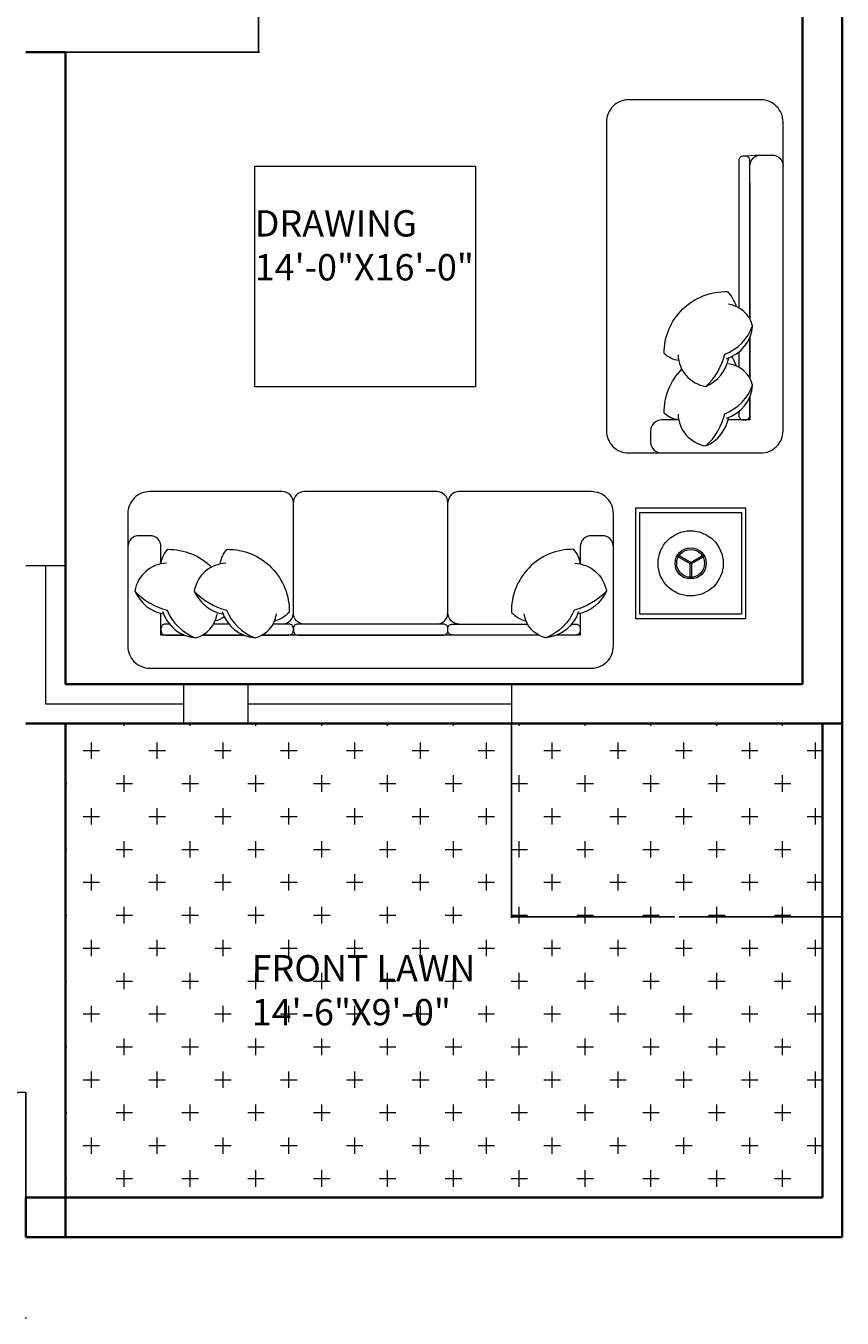
# Model space of a CAD drawing. Units: inches. Extents: x -10 to 502, y -868 to 56.
# Tile 8 of 14: x 272 to 458, y -789 to -495. Entities that reach past the tile are written whole.
import ezdxf

# ---------------------------------------------------------------- set-up
doc = ezdxf.new("R2010")
doc.units = ezdxf.units.IN
doc.header["$MEASUREMENT"] = 0
for name, color, linetype, lineweight in [('A-ANNO-DIMS', 2, 'Continuous', 18), ('A-AREA-IDEN', 7, 'Continuous', 18), ('A-FURN', 8, 'Continuous', 13), ('A-GLAZ', 162, 'Continuous', 18), ('A-WALL', 7, 'Continuous', 35), ('L-GATE', 4, 'Continuous', 25), ('L-PLNT-PATT', 101, 'Continuous', 13), ('L-WALL', 7, 'Continuous', 35)]:
    doc.layers.add(name, color=color, linetype=linetype, lineweight=lineweight)
doc.styles.get("Standard").update_dxf_attribs({"font": 'arial.ttf'})
doc.dimstyles.get("Standard").update_dxf_attribs({"dimtxt": 0.18, "dimasz": 0.18, "dimexe": 0.18, "dimexo": 0.0625, "dimgap": 0.09, "dimtad": 0, "dimtih": 1, "dimtoh": 1, "dimdec": 0, "dimzin": 0, "dimdsep": 46, "dimlunit": 3, "dimtxsty": 'Standard', "dimcen": 0.09, "dimadec": 0, "dimazin": 0, "dimtfac": 1, "dimtdec": 0, "dimtofl": 0, "dimtmove": 0, "dimatfit": 3, "dimfxl": 1, "dimtolj": 1, "dimtzin": 0, "dimarcsym": 0})

# ---------------------------------------------------------------- blocks, each defined once
blk = doc.blocks.new('WIN-60IN')
for p, q in [((0, 9), (60, 9)), ((0, 0), (0, 9)), ((60, 9), (60, 0)), ((0, 4.5), (60, 4.5)), ((60, 0), (0, 0))]:
    blk.add_line(p, q)
blk = doc.blocks.new('*D51')
at = {"layer": 'A-ANNO-DIMS', "color": 0, "lineweight": -2, "transparency": 16777216}
for p, q in [((382.59, -653.92), (382.59, -698.08)), ((457.95, -653.92), (457.95, -698.08)), ((382.77, -697.9), (419.73, -697.9)), ((457.77, -697.9), (420.81, -697.9))]:
    blk.add_line(p, q, dxfattribs=at)
at = {"layer": 'A-ANNO-DIMS', "color": 0, "transparency": 16777216}
for points in [[(382.77, -697.87), (382.77, -697.93), (382.59, -697.9)], [(457.77, -697.87), (457.77, -697.93), (457.95, -697.9)]]:
    blk.add_solid(points, dxfattribs=at)
at = {"layer": 'Defpoints', "color": 0, "transparency": 16777216}
for p in [(382.59, -653.85), (457.95, -653.85), (382.59, -697.9)]:
    blk.add_point(p, dxfattribs=at)
at = {"layer": 'A-ANNO-DIMS', "color": 0, "transparency": 16777216, "insert": (420.27, -697.9), "char_height": 0.18, "attachment_point": 5}
blk.add_mtext('\\A1;6\'-3 1/2"', dxfattribs=at)
blk = doc.blocks.new('*D58')
at = {"layer": 'A-ANNO-DIMS', "color": 0, "lineweight": -2, "transparency": 16777216}
for p, q in [((281.01, -464.85), (325.18, -464.85)), ((325, -465.03), (325, -482.67)), ((325, -500.67), (325, -483.03)), ((281.01, -500.85), (325.18, -500.85))]:
    blk.add_line(p, q, dxfattribs=at)
at = {"layer": 'A-ANNO-DIMS', "color": 0, "transparency": 16777216}
for points in [[(324.97, -465.03), (325.03, -465.03), (325, -464.85)], [(324.97, -500.67), (325.03, -500.67), (325, -500.85)]]:
    blk.add_solid(points, dxfattribs=at)
at = {"layer": 'Defpoints', "color": 0, "transparency": 16777216}
for p in [(280.95, -464.85), (280.95, -500.85), (325, -500.85)]:
    blk.add_point(p, dxfattribs=at)
at = {"layer": 'A-ANNO-DIMS', "color": 0, "transparency": 16777216, "insert": (325, -482.85), "char_height": 0.18, "attachment_point": 5}
blk.add_mtext('\\A1;3\'-0"', dxfattribs=at)
blk = doc.blocks.new('*D67')
at = {"layer": 'A-ANNO-DIMS', "color": 0, "lineweight": -2, "transparency": 16777216}
for p, q in [((228.48, -719.35), (228.66, -719.35)), ((228.66, -719.35), (244.8, -745.4)), ((271.95, -789.32), (271.95, -789.14)), ((271.86, -789.23), (272.04, -789.23))]:
    blk.add_line(p, q, dxfattribs=at)
at = {"layer": 'A-ANNO-DIMS', "color": 0, "transparency": 16777216}
blk.add_solid([(244.82, -745.39), (244.77, -745.42), (244.89, -745.56)], dxfattribs=at)
at = {"layer": 'Defpoints', "color": 0, "transparency": 16777216}
for p in [(244.89, -745.56), (271.95, -789.23)]:
    blk.add_point(p, dxfattribs=at)
at = {"layer": 'A-ANNO-DIMS', "color": 0, "transparency": 16777216, "insert": (227.85, -719.35), "char_height": 0.18, "attachment_point": 5}
blk.add_mtext('\\A1;R4\'-3 1/2"', dxfattribs=at)

msp = doc.modelspace()

# ---------------------------------------------------------------- hatches: boundary and pattern name
at = {"layer": 'L-PLNT-PATT'}
h = msp.add_hatch(dxfattribs=at)
h.set_pattern_fill('CROSS', color=256, scale=30)
h.paths.add_polyline_path([(453.45, -653.85), (280.95, -653.85), (280.95, -761.85), (453.45, -761.85)])

# ---------------------------------------------------------------- linework, layer by layer
at = {"layer": 'A-FURN'}
for p, q in [((439.45, -524.29), (435.68, -524.53)), ((423.51, -617.19), (420.44, -615.41)), ((423.35, -617.19), (426.42, -615.41)), ((423.35, -617.46), (420.28, -615.69)), ((423.27, -617.33), (423.27, -620.87)), ((423.51, -617.46), (426.58, -615.69)), ((423.59, -617.33), (423.59, -620.87))]:
    msp.add_line(p, q, dxfattribs=at)
at = {"layer": 'A-FURN', "ltscale": 0.03}
for points in [[(409.28, -511.72, 0.414214), (404.25, -516.75), (404.25, -516.75, -0.317837), (404.25, -516.75, 0.414214), (404.25, -516.75), (404.25, -516.75, -1.186185), (404.25, -516.75, 0.414214), (404.25, -516.75), (404.25, -587.15, 0.414214), (409.28, -592.18), (439.45, -592.18, 0.414214), (444.48, -587.15), (444.48, -516.75, 0.414214), (439.45, -511.72)], [(405.83, -606.01, 0.414214), (400.8, -600.98), (370.62, -600.98, 0.414214), (368.11, -603.5, 0.414214), (365.59, -600.98), (335.42, -600.98, 0.414214), (332.91, -603.5, 0.414214), (330.39, -600.98), (300.22, -600.98, 0.414214), (295.19, -606.01), (295.19, -636.18, 0.414214), (300.22, -641.21), (400.8, -641.21, 0.414214), (405.83, -636.18)]]:
    msp.add_lwpolyline(points, format="xyb", close=True, dxfattribs=at)
for points in [[(324.1, -526.8), (374.39, -526.8), (374.39, -577.09), (324.1, -577.09)], [(436, -604.75), (410.85, -604.75), (410.85, -629.9), (436, -629.9)]]:
    msp.add_lwpolyline(points, close=True, dxfattribs=at)
at = {"layer": 'A-FURN'}
for points in [[(436.93, -561.62), (436.93, -525.54, 0.414214), (435.93, -524.53), (435.43, -524.53, 0.414214), (434.42, -525.54), (434.42, -559.09, 0.414214)], [(436.93, -530.7), (436.93, -526.8, -0.414214), (439.45, -524.29), (441.96, -524.29, -0.414214), (444.48, -526.8)], [(420.72, -571.1, -0.165541), (417.39, -569.54, -0.425989), (431.8, -555.42, -0.121523), (433.78, -558.77, 7.115464)], [(431.57, -570.7, 0.306663), (437.56, -563.2, 0.30633), (432.09, -558.3, -0.872847)], [(426.9, -577.03, 0.14773), (431.22, -569.69, 0.213343), (437.56, -563.2, 0.178662)], [(436.93, -575.16), (436.93, -565.8, 0.414214)], [(420.56, -569.83, 0.356772), (426.9, -577.03, 0.249542), (432.12, -570.51, -9.61688)], [(432.8, -570.21, -0.071865), (433.78, -572.32, 7.115464)], [(434.42, -569.17), (434.42, -572.63, 0.414214)], [(420.72, -584.64, -0.165541), (417.39, -583.09, -0.200231), (421.44, -573.1, -0.121523)], [(431.57, -584.25, 0.306663), (437.56, -576.75, 0.30633), (432.09, -571.85, -0.872847)], [(426.9, -590.58, 0.14773), (431.22, -583.23, 0.213343), (437.56, -576.75, 0.178662)], [(436.93, -579.35), (436.93, -584.64), (431.99, -584.64, 0.414214)], [(436.93, -583.63), (436.93, -579.35, 0.414214)], [(434.42, -582.72), (434.42, -583.63, 0.414214), (435.43, -584.64), (435.93, -584.64, 0.414214), (436.93, -583.63)], [(420.71, -584.64), (416.82, -584.64, 0.414214), (414.3, -587.15), (414.3, -589.67, 0.414214), (416.82, -592.18)], [(420.56, -583.37, 0.356772), (426.9, -590.58, 0.249542), (432.12, -584.05, -9.61688)], [(330.39, -631.15, 0.414214), (332.91, -628.64), (332.91, -603.5, 0.41732)], [(370.62, -631.15, -0.414214), (368.11, -628.64), (368.11, -603.5, -0.415249)], [(302.73, -617.45), (302.73, -613.55, 0.414214), (300.22, -611.04), (297.7, -611.04, 0.414214), (295.19, -613.55)], [(405.83, -613.55, 0.414214), (403.31, -611.04), (400.8, -611.04, 0.414214), (398.28, -613.55), (398.28, -617.45)], [(302.73, -617.45, -0.165541), (304.28, -614.13, -0.200231), (314.26, -618.17)], [(316.27, -617.45, -0.165541), (317.83, -614.13, -0.425989), (331.95, -628.53, -0.121523), (328.6, -630.52)], [(398.29, -617.45, 0.165541), (396.73, -614.13, 0.425989), (382.61, -628.53, 0.121523), (385.96, -630.52)], [(303.99, -617.3, 0.356772), (296.79, -623.64, 0.249542), (303.32, -628.86)], [(317.54, -617.3, 0.356772), (310.33, -623.64, 0.249542), (316.86, -628.86)], [(397.02, -617.3, -0.356772), (404.23, -623.64, -0.249542), (397.7, -628.86)], [(296.79, -623.64, 0.14773), (304.14, -627.96, 0.213343), (310.62, -634.29)], [(310.33, -623.64, 0.14773), (317.68, -627.96, 0.213343), (324.17, -634.29)], [(404.23, -623.64, -0.14773), (396.88, -627.96, -0.213343), (390.39, -634.29)], [(308.02, -633.67), (302.73, -633.67), (302.73, -628.73, 0.414352)], [(303.12, -628.3, 0.306663), (310.62, -634.29, 0.30633), (315.52, -628.82)], [(317.16, -629.54, -0.071865), (315.05, -630.52)], [(316.67, -628.3, 0.306663), (324.17, -634.29, 0.30633), (329.07, -628.82)], [(335.42, -631.15, -0.414214), (332.91, -628.64)], [(365.59, -631.15, 0.414214), (368.11, -628.64)], [(397.89, -628.3, -0.306663), (390.39, -634.29, -0.30633), (385.49, -628.82)], [(304.65, -631.15), (303.74, -631.15, 0.414214), (302.73, -632.16), (302.73, -632.66, 0.414214), (303.74, -633.67)], [(318.2, -631.15), (314.74, -631.15, 0.414599)], [(325.75, -633.67), (331.9, -633.67, 0.414214), (332.91, -632.66), (332.91, -632.16, 0.414214), (331.9, -631.15), (328.28, -631.15, 0.126313)], [(388.81, -633.67), (369.11, -633.67, -0.414214), (368.11, -632.66), (368.11, -632.16, -0.414214), (369.11, -631.15), (386.28, -631.15, -0.412652)], [(396.36, -631.15), (397.28, -631.15, -0.414214), (398.28, -632.16), (398.28, -632.66, -0.414214), (397.28, -633.67)], [(303.74, -633.67), (308.02, -633.67, 0.414469)], [(312.2, -633.67), (321.57, -633.67, 0.414747)], [(397.28, -633.67), (392.99, -633.67, -0.412535)]]:
    msp.add_lwpolyline(points, format="xyb", dxfattribs=at)
for points in [[(436.93, -530.7), (436.93, -561.62)], [(436.93, -565.8), (436.93, -575.16)], [(398.28, -628.73), (398.28, -633.67), (392.99, -633.67)], [(321.57, -633.67), (312.2, -633.67)], [(388.81, -633.67), (325.75, -633.67)]]:
    msp.add_lwpolyline(points, dxfattribs=at)
msp.add_lwpolyline([(411.86, -605.76), (434.99, -605.76), (434.99, -628.89), (411.86, -628.89)], close=True, dxfattribs=at)
msp.add_lwpolyline([(333.91, -633.67), (367.1, -633.67, 0.414214), (368.11, -632.66), (368.11, -632.16, 0.414214), (367.1, -631.15), (333.91, -631.15, 0.414214), (332.91, -632.16), (332.91, -632.66, 0.414214)], format="xyb", close=True, dxfattribs=at)
for radius in [7.42, 3.55, 3.18]:
    msp.add_circle((423.43, -617.33), radius, dxfattribs=at)
at = {"layer": 'A-GLAZ'}
for p, q in [((271.95, -617.85), (280.95, -617.85)), ((276.45, -617.85), (276.45, -649.35)), ((280.95, -617.85), (280.95, -644.85)), ((280.95, -644.85), (307.95, -644.85)), ((307.95, -653.85), (307.95, -644.85)), ((276.45, -649.35), (307.95, -649.35)), ((271.95, -653.85), (307.95, -653.85))]:
    msp.add_line(p, q, dxfattribs=at)
at = {"layer": 'A-WALL'}
for p, q in [((457.95, 3.15), (457.95, -770.85)), ((448.95, -452.85), (448.95, -644.85)), ((271.95, -500.85), (280.95, -500.85)), ((280.95, -500.85), (280.95, -644.85)), ((280.95, -644.85), (448.95, -644.85)), ((271.95, -653.85), (457.95, -653.85))]:
    msp.add_line(p, q, dxfattribs=at)
at = {"layer": 'L-GATE'}
msp.add_line((271.95, -761.85), (271.95, -737.85), dxfattribs=at)
msp.add_arc((271.95, -789.23), 51.37, 90, 153.5618, dxfattribs=at)
at = {"layer": 'L-WALL'}
for p, q in [((280.95, -653.85), (280.95, -770.85)), ((453.45, -653.85), (453.45, -761.85)), ((271.95, -761.85), (271.95, -770.85)), ((271.95, -761.85), (453.45, -761.85)), ((271.95, -770.85), (457.95, -770.85))]:
    msp.add_line(p, q, dxfattribs=at)

# ---------------------------------------------------------------- block references
at = {"layer": 'A-GLAZ'}
msp.add_blockref('WIN-60IN', (322.59, -653.85), dxfattribs=at)

# ---------------------------------------------------------------- texts
at = {"layer": 'A-AREA-IDEN', "char_height": 6, "attachment_point": 1}
for s, insert in [('DRAWING\\P14\'-0"X16\'-0"', (324.1, -536.86)), ('FRONT LAWN\\P14\'-6"X9\'-0"', (323.41, -706.59))]:
    msp.add_mtext(s, dxfattribs=dict(at, insert=insert))

# ---------------------------------------------------------------- dimensions: what is measured, and where the dimension line sits
at = {"layer": 'A-ANNO-DIMS'}
for base, p1, p2, angle, picture, middle in [((325, -500.85), (280.95, -464.85), (280.95, -500.85), 270, '*D58', (325, -482.85)), ((382.59, -697.9), (457.95, -653.85), (382.59, -653.85), 180, '*D51', (420.27, -697.9))]:
    dim = msp.add_linear_dim(base=base, p1=p1, p2=p2, angle=angle, dimstyle='Standard', override={"dimdec": 1, "dimlfac": 1, "dimrnd": 0, "dimzin": 1, "dimdsep": 46, "dimlunit": 4, "dimfrac": 2}, dxfattribs=at)
    dim.commit()
    dim.dimension.update_dxf_attribs({"geometry": picture, "text_midpoint": middle})
dim = msp.add_radius_dim(center=(271.95, -789.23), mpoint=(244.89, -745.56), dimstyle='Standard', override={"dimdec": 1, "dimlfac": 1, "dimrnd": 0, "dimzin": 1, "dimdsep": 46, "dimlunit": 4, "dimfrac": 2}, dxfattribs=at)
dim.commit()
dim.dimension.update_dxf_attribs({"geometry": '*D67', "text_midpoint": (227.85, -719.35), "dimtype": 164})

doc.saveas('drawing.dxf')
